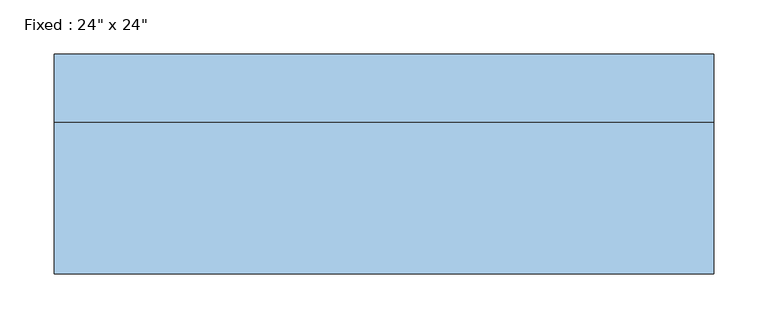
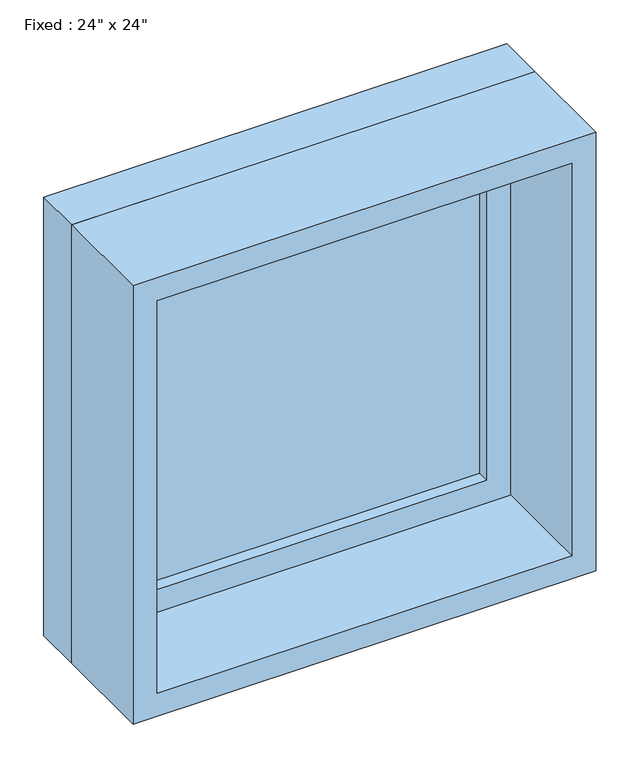
"""IFC4 building model written with IfcOpenShell, lengths in millimetres: window geometry."""

from ifc_helpers import new_model, si_unit, frame, origin, place, context, project, spatial, polyline, outline, extrude, source, transform, mapped, element, save


def window_6846e476(model_context):
    return source(origin(), model_context, "Body", "SweptSolid", [
        extrude(outline(polyline([(203.2, 53.975), (-279.4, 53.975), (-279.4, 66.675), (203.2, 66.675), (203.2, 53.975)])), frame((0.0, 0.0, 977.9), z_axis=(0.0, 0.0, 1.0), x_axis=(1.0, 0.0, 0.0)), (0.0, 0.0, 1.0), 482.6),
        extrude(outline(polyline([(1504.95, -323.85), (933.45, -323.85), (933.45, 247.65), (1504.95, 247.65), (1504.95, -323.85)]), holes=[polyline([(1460.5, -279.4), (1460.5, 203.2), (977.9, 203.2), (977.9, -279.4), (1460.5, -279.4)])]), frame((0.0, 38.1, 0.0), z_axis=(0.0, 1.0, 0.0), x_axis=(0.0, 0.0, 1.0)), (0.0, 0.0, 1.0), 44.45),
        extrude(outline(polyline([(1524.0, -342.9), (914.4, -342.9), (914.4, 266.7), (1524.0, 266.7), (1524.0, -342.9)]), holes=[polyline([(1492.25, -311.15), (1492.25, 234.95), (946.15, 234.95), (946.15, -311.15), (1492.25, -311.15)])]), frame((0.0, -101.6, 0.0), z_axis=(0.0, 1.0, 0.0), x_axis=(0.0, 0.0, 1.0)), (0.0, 0.0, 1.0), 139.7),
        extrude(outline(polyline([(1524.0, 266.7), (1524.0, -342.9), (914.4, -342.9), (914.4, 266.7), (1524.0, 266.7)]), holes=[polyline([(1504.95, 247.65), (933.45, 247.65), (933.45, -323.85), (1504.95, -323.85), (1504.95, 247.65)])]), frame((0.0, 38.1, 0.0), z_axis=(0.0, 1.0, 0.0), x_axis=(0.0, 0.0, 1.0)), (0.0, 0.0, 1.0), 63.5),
    ])


if __name__ == "__main__":
    model = new_model("IFC4")
    model_context = context("Model", 3, world=origin())
    ifc_project = project(units=[si_unit("LENGTHUNIT", "METRE", prefix="MILLI")], contexts=[model_context])
    site = spatial("IfcSite", under=ifc_project)
    building = spatial("IfcBuilding", under=site)
    placement = place(None, origin())
    window_shape = window_6846e476(model_context)
    element("IfcWindow", 1, ObjectType="Fixed : 24\" x 24\"", at=placement, inside=building, context=model_context, shape_type="MappedRepresentation", body=[
        mapped(window_shape, transform((0.0, 0.0, 0.0), x_axis=(1.0, 0.0, 0.0), y_axis=(0.0, 1.0, 0.0), z_axis=(0.0, 0.0, 1.0))),
    ])
    save(model, "model.ifc")

# Revit data of these elements
# Type "Fixed : 24\" x 24\""
#   Type Mark = "3"
#   Construction Type Id = "GSP4R"
#   Assembly Code = "B2020100"
#   Analytic Construction = "1/8 in Pilkington single glazing"
#   Visual Light Transmittance = 0.9
#   Solar Heat Gain Coefficient = 0.78
#   Heat Transfer Coefficient (U) = 0.6496 BTU/(h·ft²·°F)
#   Height = 2' - 0"
#   Default Sill Height = 3' - 0"
#   Width = 2' - 0"
#   Window Inset = 0' - 0 3/4"
#   Define Thermal Properties by = 1
#   Glass Pane Material = Glass
#   Sash Material = Sash
#   Wall Closure = (empty or 0)
# Element 1 (IfcWindow, "Fixed : 24\" x 24\"")
#   Materials on its faces: "Sash", "Glass"
# Materials
#   "Glass": class "Glass", colour RGB 0 128 192, transparency 0.75, Description = "Soda Lime Glass", Cost = 0
#   "Sash": class "Wood", colour RGB 224 178 126, transparency 0
